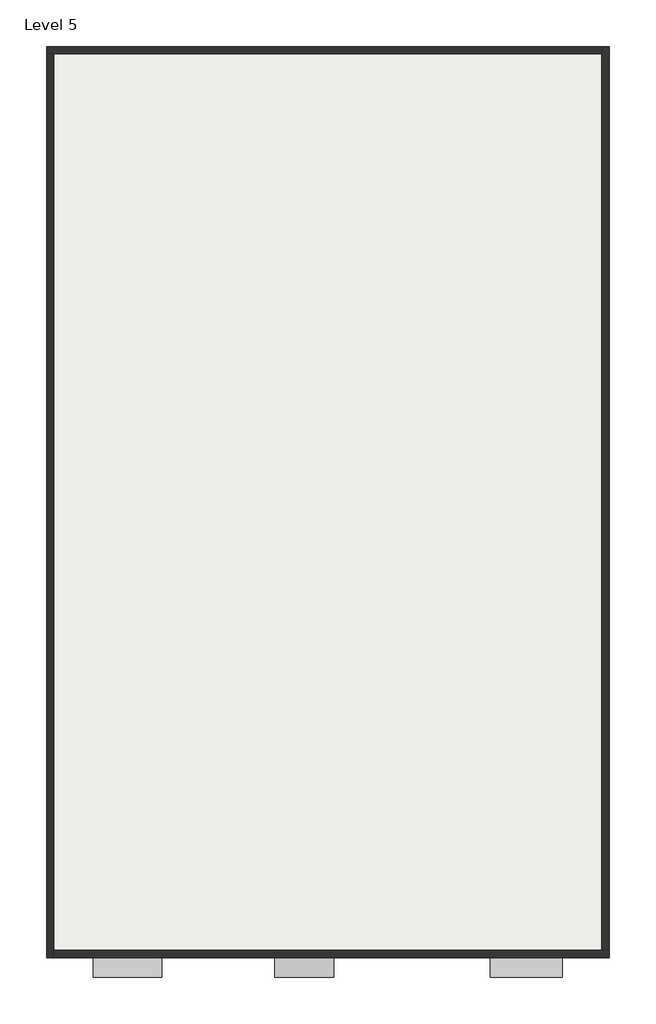
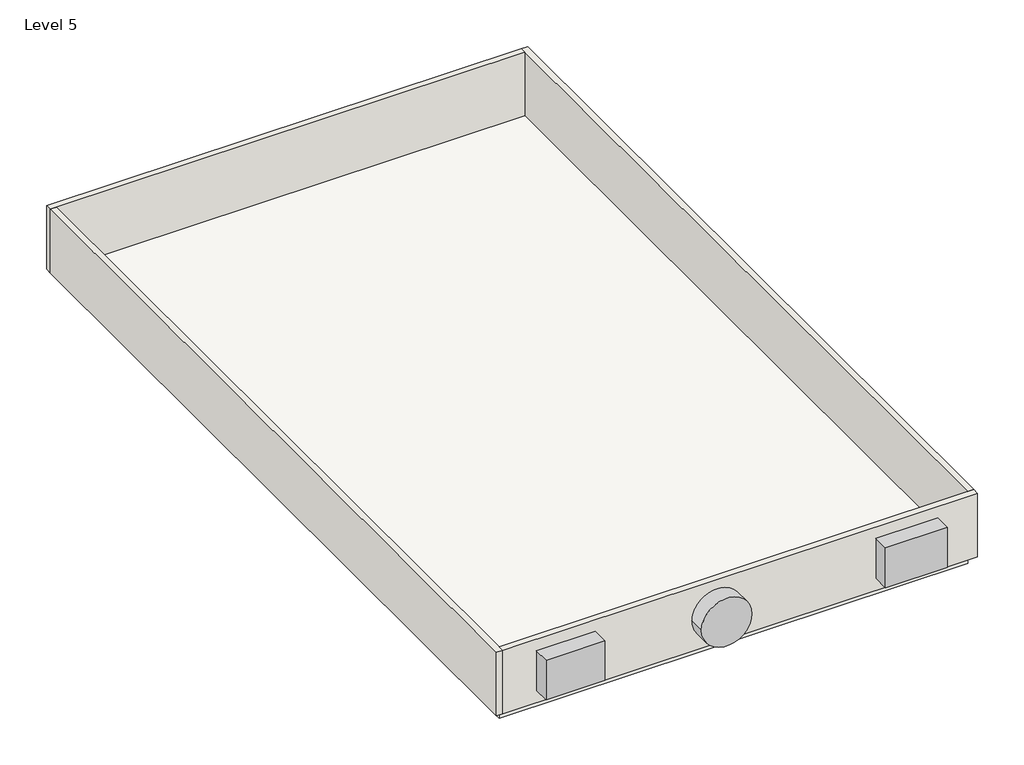
# One storey: 4 walls, 1 proxy, 1 roof.
"""IFC4 building model written with IfcOpenShell, lengths in millimetres."""

from ifc_helpers import new_model, si_unit, frame, origin, place, context, project, spatial, polyline, outline, extrude, faceted_brep, transform, mapped, element, save
from components import generic_models_5_generic_models_5_0ac3c750

model = new_model("IFC4")

# Units and contexts
model_context = context("Model", 3, world=origin())
ifc_project = project(units=[si_unit("LENGTHUNIT", "METRE", prefix="MILLI")], contexts=[model_context])

# Site, building, storey
site = spatial("IfcSite", under=ifc_project)
building = spatial("IfcBuilding", under=site)
storey = spatial("IfcBuildingStorey", under=building, Name="Level 5", Elevation=9601.2)

# Proxy
placement = place(None, origin())
generic_models_5_generic_models_5_shape = generic_models_5_generic_models_5_0ac3c750(model_context)
element("IfcBuildingElementProxy", 1, Name="Generic Models 5 : Generic Models 5", ObjectType="Generic Models 5 : Generic Models 5", at=placement, inside=storey, context=model_context, shape_type="MappedRepresentation", body=[
    mapped(generic_models_5_generic_models_5_shape, transform((0.0, 0.0, 0.0), x_axis=(1.0, 0.0, 0.0), y_axis=(0.0, 1.0, 0.0), z_axis=(0.0, 0.0, 1.0))),
])

# Roof
element("IfcRoof", 2, ObjectType="Generic - 12\"", at=placement, inside=storey, context=model_context, shape_type="SweptSolid", body=[
    extrude(outline(polyline([(-5503.3915084, 7491.4435985), (2992.9084916, 7491.4435985), (2992.9084916, -6415.0564015), (-5503.3915084, -6415.0564015), (-5503.3915084, 7491.4435985)])), frame((0.0, 0.0, 9448.8), z_axis=(0.0, 0.0, 1.0), x_axis=(1.0, 0.0, 0.0)), (0.0, 0.0, 1.0), 152.4),
])

# Walls
element("IfcWall", 3, ObjectType="WALL4.5\"", at=placement, inside=storey, context=model_context, shape_type="Brep", body=[
    faceted_brep([(-5617.6915084, 7491.4435985, 9601.2), (-5503.3915084, 7491.4435985, 9601.2), (2992.9084916, 7491.4435985, 9601.2), (2992.9084916, 7491.4435985, 10820.4), (-5503.3915084, 7491.4435985, 10820.4), (-5617.6915084, 7491.4435985, 10820.4), (-5617.6915084, 7605.7435985, 9601.2), (-5617.6915084, 7605.7435985, 10820.4), (2992.9084916, 7605.7435985, 10820.4), (2992.9084916, 7605.7435985, 9601.2)], [[[0, 1, 2, 3, 4, 5]], [[6, 7, 8, 9]], [[2, 1, 0, 6, 9]], [[5, 4, 3, 8, 7]], [[0, 5, 7, 6]], [[3, 2, 9, 8]]]),
])
element("IfcWall", 4, ObjectType="WALL4.5\"", at=placement, inside=storey, context=model_context, shape_type="Brep", body=[
    faceted_brep([(-5503.3915084, -6529.3564015, 9601.2), (-5503.3915084, -6415.0564015, 9601.2), (-5503.3915084, 7491.4435985, 9601.2), (-5503.3915084, 7491.4435985, 10820.4), (-5503.3915084, -6415.0564015, 10820.4), (-5503.3915084, -6529.3564015, 10820.4), (-5617.6915084, -6529.3564015, 9601.2), (-5617.6915084, -6529.3564015, 10820.4), (-5617.6915084, 7491.4435985, 10820.4), (-5617.6915084, 7491.4435985, 9601.2)], [[[0, 1, 2, 3, 4, 5]], [[6, 7, 8, 9]], [[2, 1, 0, 6, 9]], [[5, 4, 3, 8, 7]], [[0, 5, 7, 6]], [[3, 2, 9, 8]]]),
])
element("IfcWall", 5, ObjectType="WALL4.5\"", at=placement, inside=storey, context=model_context, shape_type="Brep", body=[
    faceted_brep([(3107.2084916, -6415.0564015, 9601.2), (2992.9084916, -6415.0564015, 9601.2), (-5503.3915084, -6415.0564015, 9601.2), (-5503.3915084, -6415.0564015, 10820.4), (2992.9084916, -6415.0564015, 10820.4), (3107.2084916, -6415.0564015, 10820.4), (3107.2084916, -6529.3564015, 9601.2), (3107.2084916, -6529.3564015, 10820.4), (-5503.3915084, -6529.3564015, 10820.4), (-5503.3915084, -6529.3564015, 9601.2)], [[[0, 1, 2, 3, 4, 5]], [[6, 7, 8, 9]], [[2, 1, 0, 6, 9]], [[5, 4, 3, 8, 7]], [[0, 5, 7, 6]], [[3, 2, 9, 8]]]),
])
element("IfcWall", 6, ObjectType="WALL4.5\"", at=placement, inside=storey, context=model_context, shape_type="Brep", body=[
    faceted_brep([(2992.9084916, 7605.7435985, 9601.2), (2992.9084916, 7491.4435985, 9601.2), (2992.9084916, -6415.0564015, 9601.2), (2992.9084916, -6415.0564015, 10820.4), (2992.9084916, 7491.4435985, 10820.4), (2992.9084916, 7605.7435985, 10820.4), (3107.2084916, 7605.7435985, 9601.2), (3107.2084916, 7605.7435985, 10820.4), (3107.2084916, -6415.0564015, 10820.4), (3107.2084916, -6415.0564015, 9601.2)], [[[0, 1, 2, 3, 4, 5]], [[6, 7, 8, 9]], [[2, 1, 0, 6, 9]], [[5, 4, 3, 8, 7]], [[0, 5, 7, 6]], [[3, 2, 9, 8]]]),
])

save(model, "model.ifc")

# Revit data of these elements
# Type "Generic - 12\""
#   Assembly Code = "B1020"
#   Layers, outside or top first: 0' - 6" no material (function 1)
# Type "WALL4.5\""
#   Assembly Code = "B2010"
#   Layers, outside or top first: 0' - 4 1/2" no material (function 1)
# Element 1 (IfcBuildingElementProxy, "Generic Models 5 : Generic Models 5")
#   Phase Created = New Construction
#   Materials on its faces: "Brick, Soldier Course"
# Element 2 (IfcRoof, "Generic - 12\"")
#   built-in parameter 1001705 = 31.5 (stored number, unit not read)
#   built-in parameter 1001701 = -0.5 (stored number, unit not read)
#   built-in parameter 1001710 = 33615
#   Phase Created = New Construction
#   Materials on its faces: "Default Roof"
# Elements 3, 4, 5, 6 (IfcWall, "WALL4.5\"")
#   Top Offset = 0' - 0"
#   Base Offset = 0' - 0"
#   Unconnected Height = 4' - 0"
#   wall height = 4' - 0"
#   Phase Created = New Construction
#   Base Constraint = Level 5
#   Materials on its faces: "Default Wall", "Wood - Stained"
# Materials
#   "Brick, Soldier Course": class "Masonry", colour RGB 170 98 104, transparency 0, Description = "Common brick soldier coursed", Cost = 0
#   "Default Roof": colour RGB 88 101 114, transparency 0, Cost = 0
#   "Default Wall": colour RGB 128 128 128, transparency 0, Cost = 0
#   "Wood - Stained": class "Wood", colour RGB 224 178 126, transparency 0, Cost = 0
